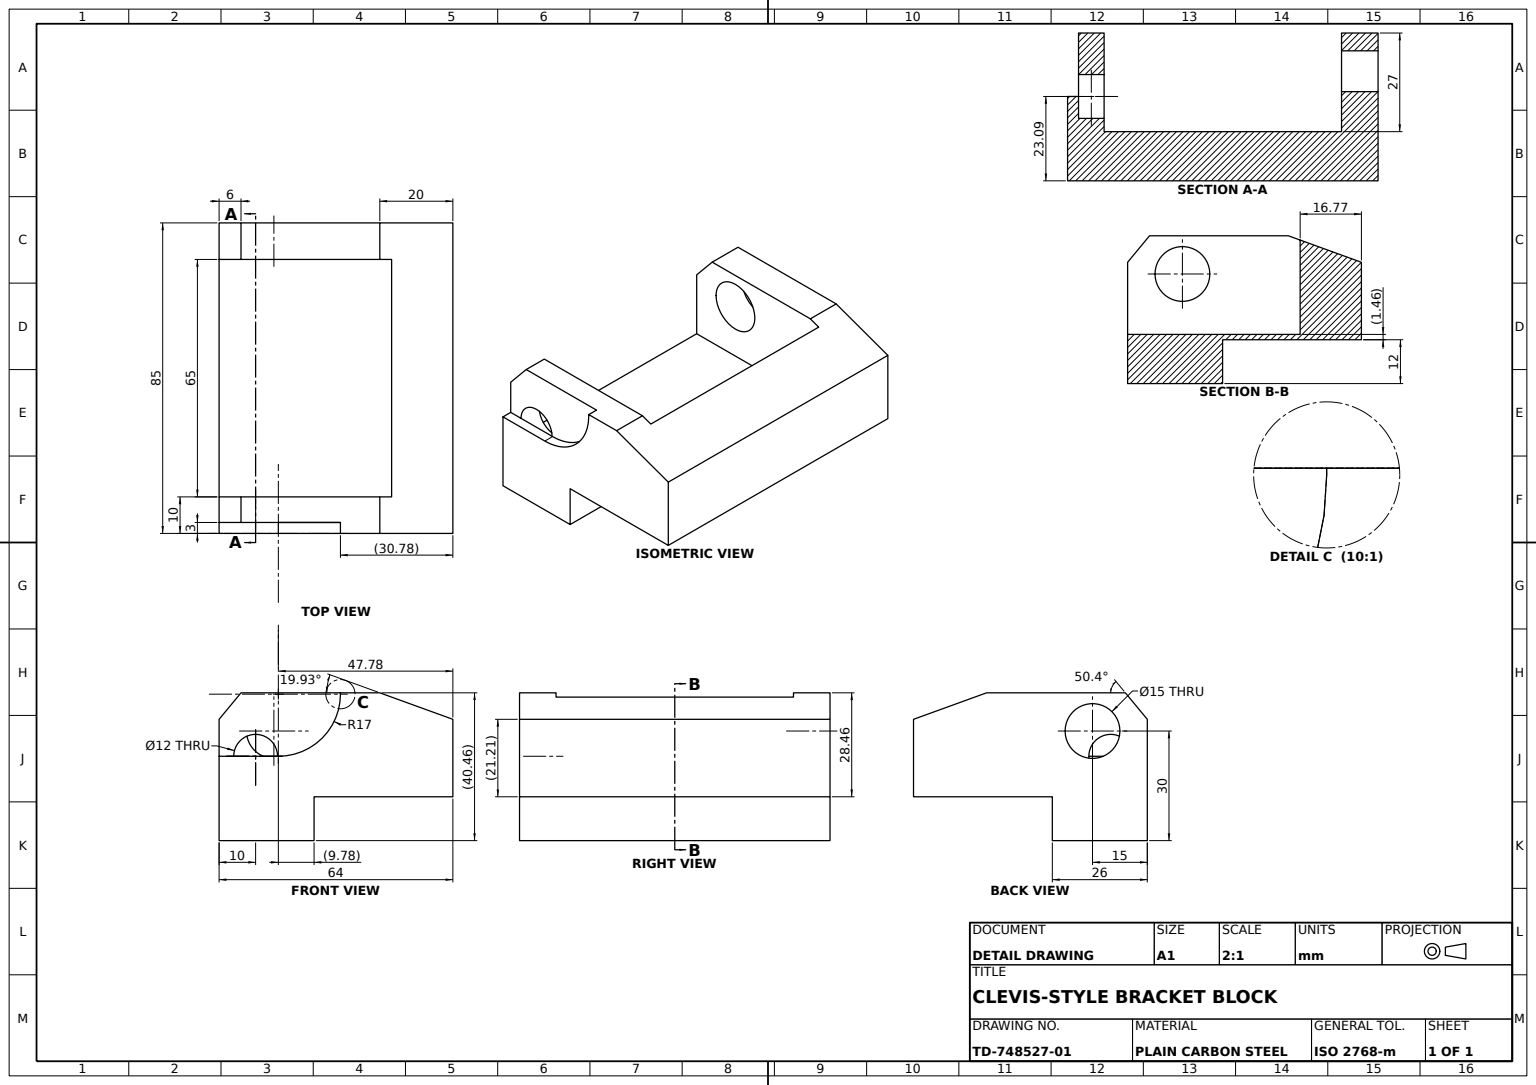
from build123d import *

# Parameters (mm, degrees)
BEARING_BLOCK_DEPTH    = 42.5
LUG_SLOT_PROFILE_W     = 65
LUG_SLOT_PROFILE_H     = 50
LUG_SLOT_65X50_DEPTH   = 27
BORE_15_SKETCH_R       = 7.5
PIVOT_BORE_15_DEPTH    = 10
LUG_RECESS_A_3MM_DEPTH = 3
LUG_RECESS_B_3MM_DEPTH = 3
BORE_10_SKETCH_R       = 6
PIVOT_BORE_10_DEPTH    = 7


with BuildPart() as part:
    # Bearing Block Profile → Bearing Block (new, symmetric)
    with BuildSketch(Plane(origin=(0, 0, 0), x_dir=(0, 0, -1), z_dir=(1, 0, 0))):
        Polygon((0, 0), (38, 0), (38, -12), (64, -12), (64, 21.206684422), (58, 28.458711219), (20, 28.458711219), (0, 21.206684422), align=None)
    extrude(amount=BEARING_BLOCK_DEPTH, both=True)

    # Lug Slot Profile → Lug Slot 65x50 (cut)
    with BuildSketch(Plane(origin=(0, 28.458711219, 0), x_dir=(1, 0, 0), z_dir=(0, 1, 0))):
        with Locations((0, 41.768401258)):
            Rectangle(LUG_SLOT_PROFILE_W, LUG_SLOT_PROFILE_H)
    extrude(amount=-LUG_SLOT_65X50_DEPTH, mode=Mode.SUBTRACT)

    # Bore Ø15 Sketch → Pivot Bore Ø15 (cut)
    with BuildSketch(Plane(origin=(42.5, 0, 0), x_dir=(0, 0, -1), z_dir=(1, 0, 0))):
        with Locations((49, 18)):
            Circle(BORE_15_SKETCH_R)
    extrude(amount=-PIVOT_BORE_15_DEPTH, mode=Mode.SUBTRACT)

    # Lug Recess A Profile → Lug Recess A 3mm (cut)
    with BuildSketch(Plane.ZY.offset(42.5)):
        with BuildLine():
            Line((-58, 28.458711219), (-63.551815655, 21.748391902))
            ThreePointArc((-63.551815655, 21.748391902), (-44.368906721, 11.436763576), (-30.783363951, 28.458711219))
            Line((-30.783363951, 28.458711219), (-58, 28.458711219))
        make_face()
    extrude(amount=-LUG_RECESS_A_3MM_DEPTH, mode=Mode.SUBTRACT)

    # Lug Recess B Profile → Lug Recess B 3mm (cut)
    with BuildSketch(Plane.ZY.offset(42.5)):
        Polygon((-47.779389931, 11.091150514), (-64, 11.091150514), (-64, 21.206684422), (-63.551815655, 21.748391902), align=None)
    extrude(amount=-LUG_RECESS_B_3MM_DEPTH, mode=Mode.SUBTRACT)

    # Bore Ø10 Sketch → Pivot Bore Ø10 (cut)
    with BuildSketch(Plane.ZY.offset(39.5)):
        with Locations(Location((-54, 11.091150514, 0), (0, 0, 180))):
            Circle(BORE_10_SKETCH_R)
    extrude(amount=-PIVOT_BORE_10_DEPTH, mode=Mode.SUBTRACT)


solid = part.part
